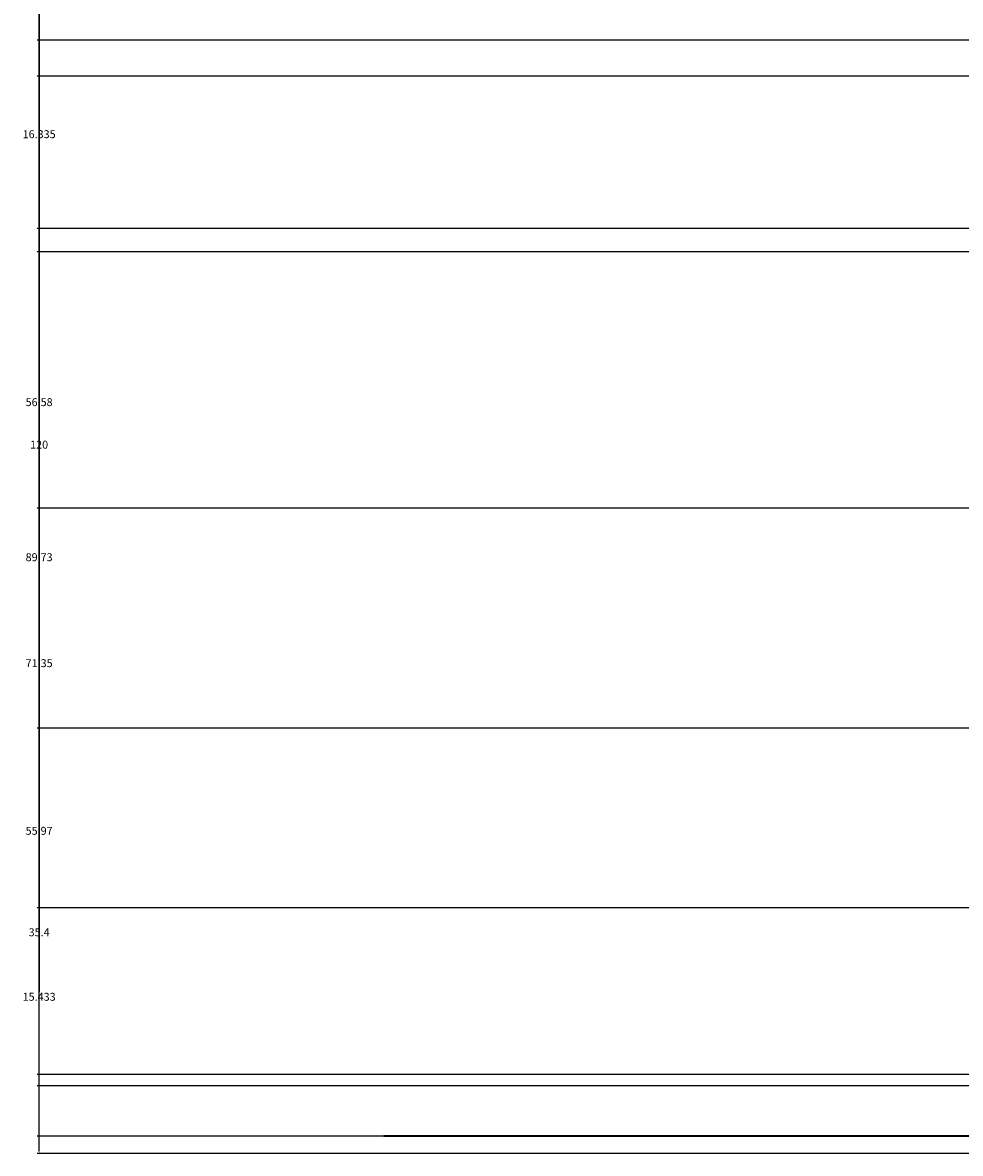
# Model space of a CAD drawing. Units: inches. Extents: x -145 to 510, y 5 to 386.
# Tile 2 of 25: x -145 to -64, y 78 to 177. Entities that reach past the tile are written whole.
import ezdxf

# ---------------------------------------------------------------- set-up
doc = ezdxf.new("R2010")
doc.units = ezdxf.units.IN
doc.header["$MEASUREMENT"] = 0
doc.layers.add('A-ANNO-DIMS', color=2, linetype='Continuous', lineweight=18)
doc.layers.add('A-ELEV', color=7, linetype='Continuous', lineweight=35)
doc.styles.get("Standard").update_dxf_attribs({"font": 'arial.ttf'})
doc.dimstyles.get("Standard").update_dxf_attribs({"dimtxt": 0.6875, "dimasz": 0.18, "dimexe": 0.18, "dimexo": 0.0625, "dimgap": 0.09, "dimtad": 0, "dimtih": 1, "dimtoh": 1, "dimdec": 4, "dimzin": 0, "dimdsep": 46, "dimlunit": 4, "dimtxsty": 'Standard', "dimcen": 0.09, "dimadec": 0, "dimazin": 0, "dimtfac": 1, "dimtdec": 4, "dimtofl": 0, "dimtmove": 0, "dimatfit": 3, "dimfxl": 1, "dimtolj": 1, "dimtzin": 0, "dimarcsym": 0})

# ---------------------------------------------------------------- blocks, each defined once
blk = doc.blocks.new('*D19')
at = {"layer": 'A-ANNO-DIMS', "color": 0, "lineweight": -2, "transparency": 16777216}
for p, q in [((478.764, 355.891), (-144.054, 355.891)), ((-143.874, 355.711), (-143.874, 218.332)), ((-143.874, 80.071), (-143.874, 217.45)), ((-114.036, 79.891), (-144.054, 79.891))]:
    blk.add_line(p, q, dxfattribs=at)
at = {"layer": 'A-ANNO-DIMS', "color": 0, "transparency": 16777216}
for points in [[(-143.904, 355.711), (-143.844, 355.711), (-143.874, 355.891)], [(-143.904, 80.071), (-143.844, 80.071), (-143.874, 79.891)]]:
    blk.add_solid(points, dxfattribs=at)
at = {"layer": 'Defpoints', "color": 0, "transparency": 16777216}
for p in [(-143.874, 355.891), (478.826, 355.891), (-113.974, 79.891)]:
    blk.add_point(p, dxfattribs=at)
at = {"layer": 'A-ANNO-DIMS', "color": 0, "transparency": 16777216, "insert": (-143.874, 217.891), "char_height": 0.6875, "attachment_point": 5}
blk.add_mtext('\\A1;276', dxfattribs=at)
blk = doc.blocks.new('*D20')
at = {"layer": 'A-ANNO-DIMS', "color": 0, "lineweight": -2, "transparency": 16777216}
for p, q in [((53.939, 199.891), (-144.054, 199.891)), ((-143.874, 199.711), (-143.874, 140.332)), ((-143.874, 80.071), (-143.874, 139.45)), ((53.939, 79.891), (-144.054, 79.891))]:
    blk.add_line(p, q, dxfattribs=at)
at = {"layer": 'A-ANNO-DIMS', "color": 0, "transparency": 16777216}
for points in [[(-143.904, 199.711), (-143.844, 199.711), (-143.874, 199.891)], [(-143.904, 80.071), (-143.844, 80.071), (-143.874, 79.891)]]:
    blk.add_solid(points, dxfattribs=at)
at = {"layer": 'Defpoints', "color": 0, "transparency": 16777216}
for p in [(-143.874, 199.891), (54.001, 199.891), (54.001, 79.891)]:
    blk.add_point(p, dxfattribs=at)
at = {"layer": 'A-ANNO-DIMS', "color": 0, "transparency": 16777216, "insert": (-143.874, 139.891), "char_height": 0.6875, "attachment_point": 5}
blk.add_mtext('\\A1;120', dxfattribs=at)
blk = doc.blocks.new('*D23')
at = {"layer": 'A-ANNO-DIMS', "color": 0, "lineweight": -2, "transparency": 16777216}
for p, q in [((88.184, 115.292), (-144.054, 115.292)), ((-143.874, 115.112), (-143.874, 98.033)), ((-143.874, 80.071), (-143.874, 97.15)), ((53.939, 79.891), (-144.054, 79.891))]:
    blk.add_line(p, q, dxfattribs=at)
at = {"layer": 'A-ANNO-DIMS', "color": 0, "transparency": 16777216}
for points in [[(-143.904, 115.112), (-143.844, 115.112), (-143.874, 115.292)], [(-143.904, 80.071), (-143.844, 80.071), (-143.874, 79.891)]]:
    blk.add_solid(points, dxfattribs=at)
at = {"layer": 'Defpoints', "color": 0, "transparency": 16777216}
for p in [(-143.874, 115.292), (88.246, 115.292), (54.001, 79.891)]:
    blk.add_point(p, dxfattribs=at)
at = {"layer": 'A-ANNO-DIMS', "color": 0, "transparency": 16777216, "insert": (-143.874, 97.591), "char_height": 0.6875, "attachment_point": 5}
blk.add_mtext('\\A1;35.4', dxfattribs=at)
blk = doc.blocks.new('*D24')
at = {"layer": 'A-ANNO-DIMS', "color": 0, "lineweight": -2, "transparency": 16777216}
for p, q in [((88.184, 171.872), (-144.054, 171.872)), ((-143.874, 171.692), (-143.874, 144.023)), ((-143.874, 115.472), (-143.874, 143.141)), ((88.184, 115.292), (-144.054, 115.292))]:
    blk.add_line(p, q, dxfattribs=at)
at = {"layer": 'A-ANNO-DIMS', "color": 0, "transparency": 16777216}
for points in [[(-143.904, 171.692), (-143.844, 171.692), (-143.874, 171.872)], [(-143.904, 115.472), (-143.844, 115.472), (-143.874, 115.292)]]:
    blk.add_solid(points, dxfattribs=at)
at = {"layer": 'Defpoints', "color": 0, "transparency": 16777216}
for p in [(-143.874, 171.872), (88.246, 171.872), (88.246, 115.292)]:
    blk.add_point(p, dxfattribs=at)
at = {"layer": 'A-ANNO-DIMS', "color": 0, "transparency": 16777216, "insert": (-143.874, 143.582), "char_height": 0.6875, "attachment_point": 5}
blk.add_mtext('\\A1;56.58', dxfattribs=at)
blk = doc.blocks.new('*D29')
at = {"layer": 'A-ANNO-DIMS', "color": 0, "lineweight": -2, "transparency": 16777216}
for p, q in [((221.467, 174.992), (-144.054, 174.992)), ((-143.874, 174.812), (-143.874, 130.569)), ((-143.874, 85.444), (-143.874, 129.687)), ((221.467, 85.264), (-144.054, 85.264))]:
    blk.add_line(p, q, dxfattribs=at)
at = {"layer": 'A-ANNO-DIMS', "color": 0, "transparency": 16777216}
for points in [[(-143.904, 174.812), (-143.844, 174.812), (-143.874, 174.992)], [(-143.904, 85.444), (-143.844, 85.444), (-143.874, 85.264)]]:
    blk.add_solid(points, dxfattribs=at)
at = {"layer": 'Defpoints', "color": 0, "transparency": 16777216}
for p in [(-143.874, 174.992), (221.529, 174.992), (221.529, 85.264)]:
    blk.add_point(p, dxfattribs=at)
at = {"layer": 'A-ANNO-DIMS', "color": 0, "transparency": 16777216, "insert": (-143.874, 130.128), "char_height": 0.6875, "attachment_point": 5}
blk.add_mtext('\\A1;89.73', dxfattribs=at)
blk = doc.blocks.new('*D42')
at = {"layer": 'A-ANNO-DIMS', "color": 0, "lineweight": -2, "transparency": 16777216}
for p, q in [((-23.036, 134.378), (-144.054, 134.378)), ((-143.874, 134.198), (-143.874, 106.835)), ((-143.874, 78.591), (-143.874, 105.953)), ((-60.445, 78.411), (-144.054, 78.411))]:
    blk.add_line(p, q, dxfattribs=at)
at = {"layer": 'A-ANNO-DIMS', "color": 0, "transparency": 16777216}
for points in [[(-143.904, 134.198), (-143.844, 134.198), (-143.874, 134.378)], [(-143.904, 78.591), (-143.844, 78.591), (-143.874, 78.411)]]:
    blk.add_solid(points, dxfattribs=at)
at = {"layer": 'Defpoints', "color": 0, "transparency": 16777216}
for p in [(-143.874, 134.378), (-22.974, 134.378), (-60.383, 78.411)]:
    blk.add_point(p, dxfattribs=at)
at = {"layer": 'A-ANNO-DIMS', "color": 0, "transparency": 16777216, "insert": (-143.874, 106.394), "char_height": 0.6875, "attachment_point": 5}
blk.add_mtext('\\A1;55.97', dxfattribs=at)
blk = doc.blocks.new('*D54')
at = {"layer": 'A-ANNO-DIMS', "color": 0, "lineweight": -2, "transparency": 16777216}
for p, q in [((315.492, 156.609), (-144.054, 156.609)), ((-143.874, 156.429), (-143.874, 121.378)), ((-143.874, 85.444), (-143.874, 120.495)), ((315.492, 85.264), (-144.054, 85.264))]:
    blk.add_line(p, q, dxfattribs=at)
at = {"layer": 'A-ANNO-DIMS', "color": 0, "transparency": 16777216}
for points in [[(-143.904, 156.429), (-143.844, 156.429), (-143.874, 156.609)], [(-143.904, 85.444), (-143.844, 85.444), (-143.874, 85.264)]]:
    blk.add_solid(points, dxfattribs=at)
at = {"layer": 'Defpoints', "color": 0, "transparency": 16777216}
for p in [(-143.874, 156.609), (315.554, 156.609), (315.554, 85.264)]:
    blk.add_point(p, dxfattribs=at)
at = {"layer": 'A-ANNO-DIMS', "color": 0, "transparency": 16777216, "insert": (-143.874, 120.937), "char_height": 0.6875, "attachment_point": 5}
blk.add_mtext('\\A1;71.35', dxfattribs=at)
blk = doc.blocks.new('*D55')
at = {"layer": 'A-ANNO-DIMS', "color": 0, "lineweight": -2, "transparency": 16777216}
for p, q in [((314.432, 174.992), (-144.054, 174.992)), ((-143.874, 174.812), (-143.874, 167.266)), ((-143.874, 158.837), (-143.874, 166.383)), ((314.432, 158.657), (-144.054, 158.657))]:
    blk.add_line(p, q, dxfattribs=at)
at = {"layer": 'A-ANNO-DIMS', "color": 0, "transparency": 16777216}
for points in [[(-143.904, 174.812), (-143.844, 174.812), (-143.874, 174.992)], [(-143.904, 158.837), (-143.844, 158.837), (-143.874, 158.657)]]:
    blk.add_solid(points, dxfattribs=at)
at = {"layer": 'Defpoints', "color": 0, "transparency": 16777216}
for p in [(-143.874, 174.992), (314.494, 174.992), (314.494, 158.657)]:
    blk.add_point(p, dxfattribs=at)
at = {"layer": 'A-ANNO-DIMS', "color": 0, "transparency": 16777216, "insert": (-143.874, 166.825), "char_height": 0.6875, "attachment_point": 5}
blk.add_mtext('\\A1;16.335', dxfattribs=at)
blk = doc.blocks.new('*D57')
at = {"layer": 'A-ANNO-DIMS', "color": 0, "lineweight": -2, "transparency": 16777216}
for p, q in [((263.856, 99.712), (-144.054, 99.712)), ((-143.874, 99.532), (-143.874, 92.436)), ((-143.874, 84.459), (-143.874, 91.554)), ((271.428, 84.279), (-144.054, 84.279))]:
    blk.add_line(p, q, dxfattribs=at)
at = {"layer": 'A-ANNO-DIMS', "color": 0, "transparency": 16777216}
for points in [[(-143.904, 99.532), (-143.844, 99.532), (-143.874, 99.712)], [(-143.904, 84.459), (-143.844, 84.459), (-143.874, 84.279)]]:
    blk.add_solid(points, dxfattribs=at)
at = {"layer": 'Defpoints', "color": 0, "transparency": 16777216}
for p in [(-143.874, 99.712), (263.918, 99.712), (271.491, 84.279)]:
    blk.add_point(p, dxfattribs=at)
at = {"layer": 'A-ANNO-DIMS', "color": 0, "transparency": 16777216, "insert": (-143.874, 91.995), "char_height": 0.6875, "attachment_point": 5}
blk.add_mtext('\\A1;15.433', dxfattribs=at)

msp = doc.modelspace()

# ---------------------------------------------------------------- linework, layer by layer
at = {"layer": 'A-ELEV'}
msp.add_line((54.0014, 79.8905), (-113.9737, 79.8905), dxfattribs=at)

# ---------------------------------------------------------------- dimensions: what is measured, and where the dimension line sits
at = {"layer": 'A-ANNO-DIMS'}
for base, p1, p2, override, picture, middle in [((-143.8737, 355.8905), (-113.9737, 79.8905), (478.8263, 355.8905), {"dimdec": 0, "dimlfac": 1, "dimrnd": 0, "dimzin": 0, "dimdsep": 46, "dimlunit": 2}, '*D19', (-143.8737, 217.8905)), ((-143.8737, 199.8905), (54.0014, 79.8905), (54.0014, 199.8905), {"dimdec": 0, "dimlfac": 1, "dimrnd": 0, "dimzin": 0, "dimdsep": 46, "dimlunit": 2}, '*D20', (-143.8737, 139.8905)), ((-143.8737, 174.9923), (314.494, 158.657), (314.494, 174.9923), {"dimdec": 3, "dimlfac": 1, "dimrnd": 0, "dimzin": 0, "dimdsep": 46, "dimlunit": 2}, '*D55', (-143.8737, 166.8247)), ((-143.8737, 174.9923), (221.5292, 85.2638), (221.5292, 174.9923), {"dimdec": 2, "dimlfac": 1, "dimrnd": 0, "dimzin": 0, "dimdsep": 46, "dimlunit": 2}, '*D29', (-143.8737, 130.1281)), ((-143.8737, 171.8717), (88.2462, 115.2922), (88.2462, 171.8717), {"dimdec": 2, "dimlfac": 1, "dimrnd": 0, "dimzin": 0, "dimdsep": 46, "dimlunit": 2}, '*D24', (-143.8737, 143.5819)), ((-143.8737, 156.6093), (315.5545, 85.2638), (315.5545, 156.6093), {"dimdec": 2, "dimlfac": 1, "dimrnd": 0, "dimzin": 0, "dimdsep": 46, "dimlunit": 2}, '*D54', (-143.8737, 120.9365)), ((-143.8737, 134.3781), (-60.3826, 78.4107), (-22.9739, 134.3781), {"dimdec": 2, "dimlfac": 1, "dimrnd": 0, "dimzin": 0, "dimdsep": 46, "dimlunit": 2}, '*D42', (-143.8737, 106.3944)), ((-143.8737, 115.2922), (54.0014, 79.8905), (88.2462, 115.2922), {"dimdec": 1, "dimlfac": 1, "dimrnd": 0, "dimzin": 0, "dimdsep": 46, "dimlunit": 2}, '*D23', (-143.8737, 97.5914)), ((-143.8737, 99.7118), (271.4905, 84.2785), (263.9183, 99.7118), {"dimdec": 3, "dimlfac": 1, "dimrnd": 0, "dimzin": 0, "dimdsep": 46, "dimlunit": 2}, '*D57', (-143.8737, 91.9952))]:
    dim = msp.add_linear_dim(base=base, p1=p1, p2=p2, angle=90, dimstyle='Standard', override=override, dxfattribs=at)
    dim.commit()
    dim.dimension.update_dxf_attribs({"geometry": picture, "text_midpoint": middle})

doc.saveas('drawing.dxf')
